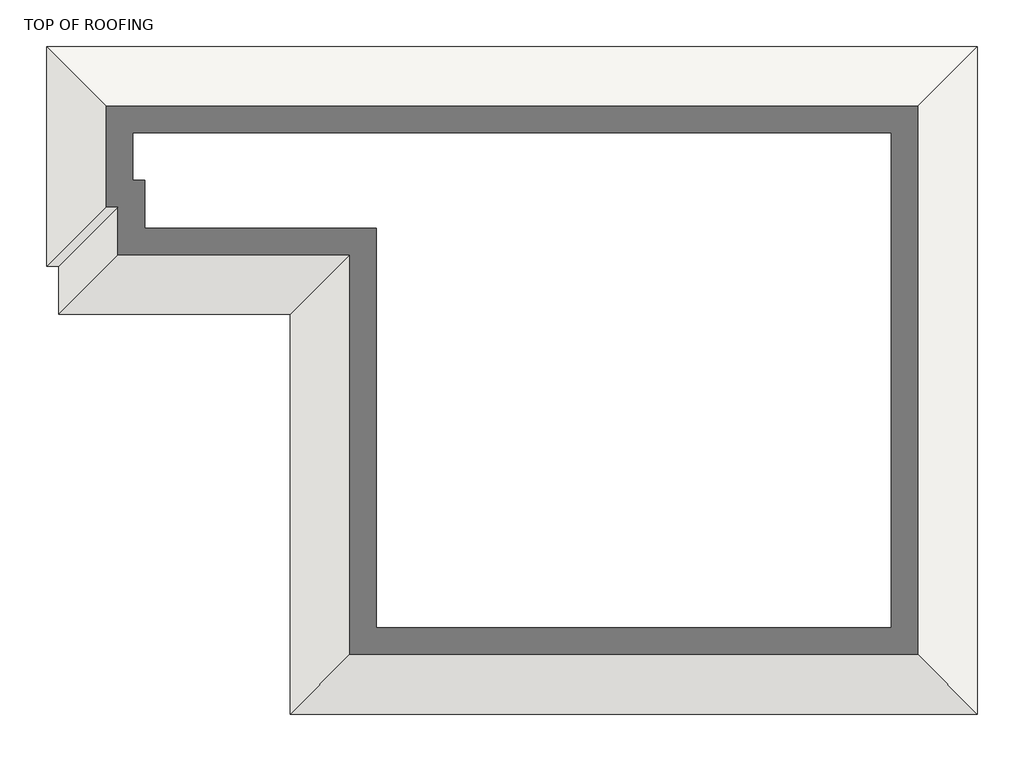
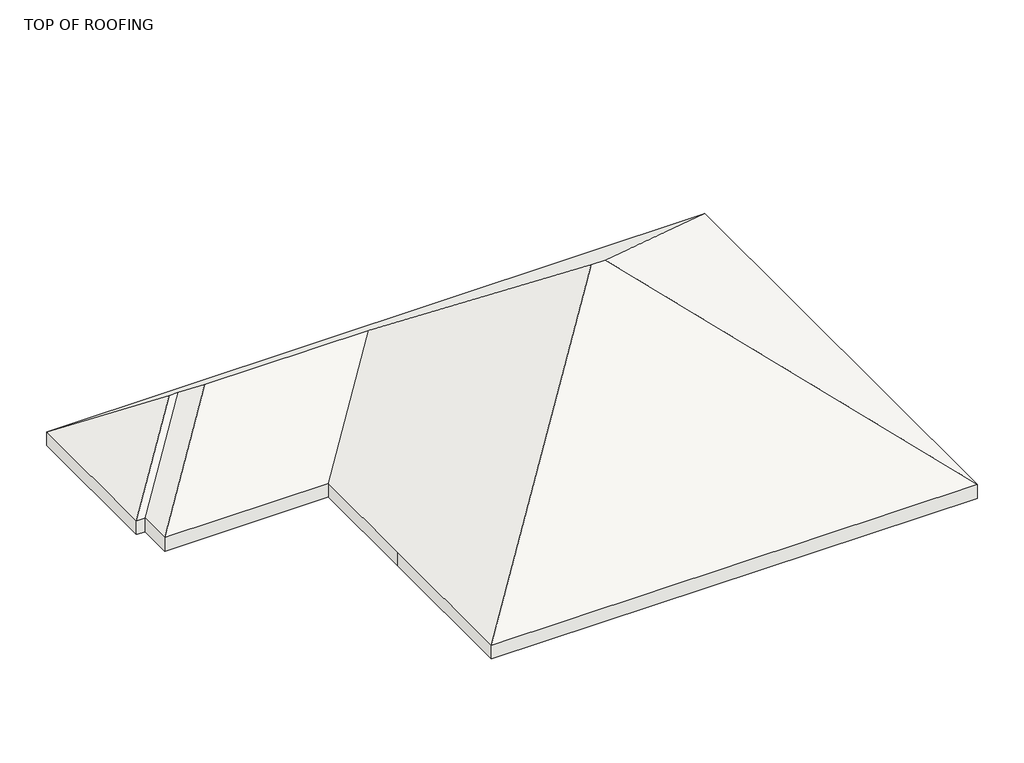
# One storey: 1 roof.
"""IFC4 building model written with IfcOpenShell, lengths in millimetres."""

from ifc_helpers import new_model, si_unit, origin, place, context, project, spatial, faceted_brep, element, save

model = new_model("IFC4")

# Units and contexts
model_context = context("Model", 3, world=origin())
ifc_project = project(units=[si_unit("LENGTHUNIT", "METRE", prefix="MILLI")], contexts=[model_context])

# Site, building, storey
site = spatial("IfcSite", under=ifc_project)
building = spatial("IfcBuilding", under=site)
storey = spatial("IfcBuildingStorey", under=building, Name="TOP OF ROOFING", Elevation=9144.0)

# Roof
placement = place(None, origin())
element("IfcRoof", 1, ObjectType="Generic - 12\"", at=placement, inside=storey, context=model_context, shape_type="Brep", body=[
    faceted_brep([(-5802.968323, 12517.59348, 9144.0), (-5802.968323, 16583.3356247, 9144.0), (-3770.0972506, 14550.4645524, 10668.6533043), (-5574.368323, 12517.59348, 9144.0), (-3541.4972506, 14550.4645524, 10668.6533043), (-3096.9972506, 14105.9645524, 11002.0283043), (-5574.368323, 11628.59348, 9144.0), (1181.4175609, 14105.9645524, 11002.0283043), (-1295.9535114, 11628.59348, 9144.0), (4876.2464886, 10411.1356247, 13773.15), (-1295.9535114, 4238.9356247, 9144.0), (-1295.9535114, 8506.1356247, 9144.0), (5241.8141504, 10411.1356247, 13773.15), (11414.0141504, 4238.9356247, 9144.0), (11414.0141504, 16583.3356247, 9144.0), (-5802.968323, 12517.59348, 9525.0), (-3770.0972506, 14550.4645524, 11049.6533043), (-5802.968323, 16583.3356247, 9525.0), (-5574.368323, 12517.59348, 9525.0), (-3541.4972506, 14550.4645524, 11049.6533043), (-5574.368323, 11628.59348, 9525.0), (-3096.9972506, 14105.9645524, 11383.0283043), (-1295.9535114, 11628.59348, 9525.0), (1181.4175609, 14105.9645524, 11383.0283043), (-1295.9535114, 8506.1356247, 9525.0), (-1295.9535114, 4238.9356247, 9525.0), (4876.2464886, 10411.1356247, 14154.15), (11414.0141504, 4238.9356247, 9525.0), (5241.8141504, 10411.1356247, 14154.15), (11414.0141504, 16583.3356247, 9525.0)], [[[0, 1, 2]], [[3, 0, 2, 4]], [[3, 4, 5, 6]], [[6, 5, 7, 8]], [[8, 7, 9, 10, 11]], [[10, 9, 12, 13]], [[13, 12, 14]], [[14, 12, 9, 7, 5, 4, 2, 1]], [[15, 16, 17]], [[15, 18, 19, 16]], [[18, 20, 21, 19]], [[20, 22, 23, 21]], [[22, 24, 25, 26, 23]], [[25, 27, 28, 26]], [[27, 29, 28]], [[29, 17, 16, 19, 21, 23, 26, 28]], [[3, 18, 15, 0]], [[6, 20, 18, 3]], [[8, 22, 20, 6]], [[11, 24, 22, 8]], [[10, 25, 24, 11]], [[13, 27, 25, 10]], [[14, 29, 27, 13]], [[1, 17, 29, 14]], [[0, 15, 17, 1]]]),
])

save(model, "model.ifc")

# Revit data of these elements
# Type "Generic - 12\""
#   Assembly Code = "B1020"
#   Layers, outside or top first: 1' - 0" no material (function 1)
# Element 1 (IfcRoof, "Generic - 12\"")
#   built-in parameter 1001705 = 46.4375 (stored number, unit not read)
#   built-in parameter 1001710 = 33615
#   Phase Created = New Construction
#   Materials on its faces: "Default Roof"
# Materials
#   "Default Roof": colour RGB 88 101 114, transparency 0, Cost = 0
